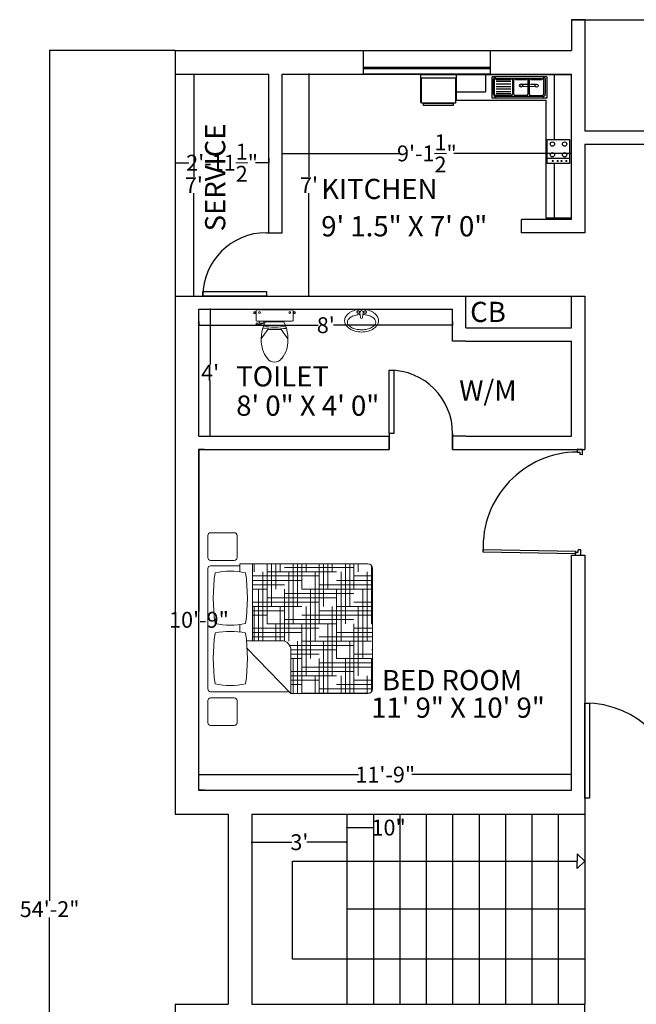
# Model space of a CAD drawing. Units: inches. Extents: x -113 to 5399, y -1393 to 3302.
# Tile 15 of 40: x 1545 to 1779, y 426 to 798. Entities that reach past the tile are written whole.
import ezdxf

# ---------------------------------------------------------------- set-up
doc = ezdxf.new("R2010")
doc.units = ezdxf.units.IN
doc.header["$MEASUREMENT"] = 0
for name, color, linetype, lineweight in [('A-ANNO-DIMS', 254, 'Continuous', 18), ('A-AREA-IDEN', 4, 'Continuous', 18), ('A-FLOR-CASE', 8, 'Continuous', 18), ('A-FLOR-FIXT', 8, 'Continuous', 18), ('doors', 2, 'Continuous', 25), ('DT TEXT', 4, 'Continuous', 18), ('furniture', 131, 'Continuous', 18), ('stairs', 210, 'Continuous', 25), ('walls', 1, 'Continuous', 25), ('windows', 3, 'Continuous', 25)]:
    doc.layers.add(name, color=color, linetype=linetype, lineweight=lineweight)
doc.layers.add('TEFRIŞ', color=11, linetype='Continuous')
doc.styles.get("Standard").update_dxf_attribs({"font": 'arial.ttf'})
doc.dimstyles.get("Standard").update_dxf_attribs({"dimtxt": 6, "dimasz": 0.18, "dimexe": 0.18, "dimexo": 0.0625, "dimgap": 0.09, "dimtad": 0, "dimtih": 1, "dimtoh": 1, "dimdec": 1, "dimzin": 0, "dimdsep": 46, "dimlunit": 4, "dimtxsty": 'Standard', "dimblk": 'ARCHTICK', "dimcen": 0.09, "dimadec": 0, "dimazin": 0, "dimtfac": 1, "dimtdec": 1, "dimtofl": 0, "dimtmove": 0, "dimatfit": 3, "dimfxl": 1, "dimtolj": 1, "dimtzin": 0, "dimarcsym": 0})

# ---------------------------------------------------------------- blocks, each defined once
blk = doc.blocks.new('*U2')
for p, q in [((0, 0), (0, -6)), ((24, 0), (24, -6))]:
    blk.add_line(p, q)
blk.add_lwpolyline([(0, 0), (0, 24), (1.75, 24), (1.75, 0)], close=True)
blk.add_arc((0, 0), 24, 0, 90)
blk = doc.blocks.new('*U3')
for p, q in [((0, 0), (0, -6)), ((36, 0), (36, -6))]:
    blk.add_line(p, q)
blk.add_lwpolyline([(0, 0), (0, 36), (1.75, 36), (1.75, 0)], close=True)
blk.add_arc((0, 0), 36, 0, 90)
blk = doc.blocks.new('*X4')
at = {"color": 0}
for p, q in [((4.359, 18.562), (4.359, 18.646)), ((4.5, 18), (4.5, 18.646)), ((4.547, 18.188), (4.547, 18.646)), ((4.594, 18.375), (4.594, 18.646)), ((4.641, 18.562), (4.641, 18.646)), ((4.781, 18), (4.781, 18.646)), ((4.828, 18.188), (4.828, 18.646)), ((4.875, 18.375), (4.875, 18.646)), ((4.922, 18.562), (4.922, 18.646)), ((5.062, 18), (5.062, 18.646)), ((5.109, 18.188), (5.109, 18.646)), ((5.156, 18.375), (5.156, 18.646)), ((5.203, 18.562), (5.203, 18.646)), ((5.344, 18), (5.344, 18.646)), ((5.391, 18.188), (5.391, 18.646)), ((5.437, 18.375), (5.437, 18.646)), ((5.484, 18.562), (5.484, 18.646)), ((5.625, 18), (5.625, 18.629)), ((4.34, 18.516), (5.062, 18.516)), ((4.453, 17.817), (4.453, 18.562)), ((4.5, 18.562), (5.25, 18.562)), ((4.687, 18.609), (5.437, 18.609)), ((4.734, 17.812), (4.734, 18.562)), ((5.016, 17.812), (5.016, 18.562)), ((5.297, 17.812), (5.297, 18.562)), ((5.437, 18.516), (5.637, 18.516)), ((5.578, 17.812), (5.578, 18.562)), ((5.625, 18.562), (5.637, 18.562)), ((4.34, 18.469), (4.875, 18.469)), ((4.34, 18.422), (4.687, 18.422)), ((5.062, 18.422), (5.637, 18.422)), ((5.25, 18.469), (5.637, 18.469)), ((4.34, 18.375), (4.5, 18.375)), ((4.406, 17.817), (4.406, 18.375)), ((4.687, 18.328), (5.437, 18.328)), ((4.687, 17.811), (4.687, 18.375)), ((4.875, 18.375), (5.625, 18.375)), ((4.969, 17.625), (4.969, 18.375)), ((5.25, 17.625), (5.25, 18.375)), ((5.531, 17.625), (5.531, 18.375)), ((4.34, 18.234), (5.062, 18.234)), ((4.5, 18.281), (5.25, 18.281)), ((5.437, 18.234), (5.637, 18.234)), ((5.625, 18.281), (5.637, 18.281)), ((4.34, 18.188), (4.875, 18.188)), ((4.34, 18.141), (4.687, 18.141)), ((4.34, 18.094), (4.5, 18.094)), ((4.359, 17.817), (4.359, 18.188)), ((4.641, 17.817), (4.641, 18.188)), ((4.875, 18.094), (5.625, 18.094)), ((4.922, 17.438), (4.922, 18.188)), ((5.062, 18.141), (5.637, 18.141)), ((5.203, 17.438), (5.203, 18.188)), ((5.25, 18.188), (5.637, 18.188)), ((5.484, 17.438), (5.484, 18.188)), ((4.5, 18), (5.25, 18)), ((4.594, 17.817), (4.594, 18)), ((4.687, 18.047), (5.437, 18.047)), ((4.875, 17.25), (4.875, 18)), ((5.156, 17.25), (5.156, 18)), ((5.437, 17.25), (5.437, 18)), ((5.625, 18), (5.637, 18)), ((4.34, 17.953), (5.062, 17.953)), ((4.34, 17.906), (4.875, 17.906)), ((5.25, 17.906), (5.637, 17.906)), ((5.437, 17.953), (5.637, 17.953)), ((4.34, 17.859), (4.687, 17.859)), ((4.828, 17.246), (4.828, 17.812)), ((4.875, 17.812), (5.625, 17.812)), ((5.062, 17.859), (5.637, 17.859)), ((5.109, 17.246), (5.109, 17.812)), ((5.391, 17.246), (5.391, 17.812)), ((4.742, 17.766), (5.437, 17.766)), ((4.755, 17.719), (5.25, 17.719)), ((4.755, 17.672), (5.062, 17.672)), ((5.437, 17.672), (5.637, 17.672)), ((5.625, 17.719), (5.637, 17.719)), ((4.755, 17.625), (4.875, 17.625)), ((4.781, 17.246), (4.781, 17.625)), ((5.062, 17.246), (5.062, 17.625)), ((5.062, 17.578), (5.637, 17.578)), ((5.25, 17.625), (5.637, 17.625)), ((5.344, 17.246), (5.344, 17.625)), ((5.625, 17.263), (5.625, 17.625)), ((4.755, 17.484), (5.437, 17.484)), ((4.875, 17.531), (5.625, 17.531)), ((4.755, 17.438), (5.25, 17.438)), ((4.755, 17.391), (5.062, 17.391)), ((4.755, 17.344), (4.875, 17.344)), ((5.016, 17.246), (5.016, 17.438)), ((5.25, 17.344), (5.637, 17.344)), ((5.297, 17.246), (5.297, 17.438)), ((5.437, 17.391), (5.637, 17.391)), ((5.578, 17.246), (5.578, 17.438)), ((5.625, 17.438), (5.637, 17.438)), ((4.875, 17.25), (5.608, 17.25)), ((4.969, 17.246), (4.969, 17.25)), ((5.062, 17.297), (5.637, 17.297)), ((5.25, 17.246), (5.25, 17.25)), ((5.531, 17.246), (5.531, 17.25))]:
    blk.add_line(p, q, dxfattribs=at)
blk = doc.blocks.new('MAT-P01')
for p, q in [((-0.021, 0.816), (-0.021, 0.56)), ((0.009, 0.846), (0.247, 0.846)), ((0.277, 0.816), (0.277, 0.56)), ((0.344, 0.816), (0.344, -0.032)), ((0.374, 0.846), (1.674, 0.846)), ((1.704, 0.816), (1.704, 0.5)), ((1.762, 0.816), (1.762, 0.56)), ((1.792, 0.846), (2.031, 0.846)), ((2.061, 0.816), (2.061, 0.56)), ((0.009, 0.53), (0.247, 0.53)), ((0.895, 0.429), (0.895, 0.049)), ((0.988, 0.5), (1.069, 0.5)), ((1.639, 0.5), (1.724, 0.5)), ((1.724, 0.5), (1.724, -0.884)), ((1.792, 0.53), (2.031, 0.53)), ((0.815, 0.423), (0.324, -0.051)), ((0.895, 0.364), (1.724, 0.364)), ((0.895, 0.364), (0.895, 0.049)), ((0.895, 0.364), (1.724, 0.364)), ((1.724, 0.364), (1.724, -0.884)), ((0.324, -0.051), (0.795, -0.051)), ((0.324, -0.051), (0.324, -0.884)), ((0.374, -0.934), (1.674, -0.934))]:
    blk.add_line(p, q)
for centre, radius, start, end in [((0.009, 0.816), 0.03, 90, 180), ((0.247, 0.816), 0.03, 0, 90), ((0.374, 0.816), 0.03, 90, 180), ((1.225, 0.603), 0.814, 168.373, 191.627), ((0.703, -1.144), 1.931, 81.8162, 98.1838), ((0.181, 0.603), 0.814, 348.373, 11.627), ((1.877, 0.603), 0.814, 168.373, 191.627), ((1.354, -1.144), 1.931, 81.8162, 98.1838), ((0.832, 0.603), 0.814, 348.373, 11.627), ((1.674, 0.816), 0.03, 0, 90), ((1.792, 0.816), 0.03, 90, 180), ((2.031, 0.816), 0.03, 0, 90), ((0.009, 0.56), 0.03, 180, 270), ((0.247, 0.56), 0.03, 270, 0), ((1.792, 0.56), 0.03, 180, 270), ((2.031, 0.56), 0.03, 270, 0), ((0.703, 2.35), 1.931, 261.8162, 278.1838), ((1.354, 2.35), 1.931, 261.8162, 278.1838), ((0.795, 0.049), 0.1, 270, 0), ((0.374, -0.884), 0.05, 180, 270), ((1.674, -0.884), 0.05, 270, 0)]:
    blk.add_arc(centre, radius, start, end)
at = {"rotation": 270}
blk.add_blockref('*X4', (-16.922, 4.704), dxfattribs=at)
blk = doc.blocks.new('A$C008029BD')
at = {"layer": 'TEFRIŞ', "ltscale": 0.05}
for p, q in [((0, 0), (0, -3.55)), ((3.37, 0), (0, 0)), ((3.37, 0), (3.37, -0.6)), ((1.522, -0.4), (0, -0.4)), ((3.37, -0.4), (2.083, -0.4)), ((0.05, -0.581), (0.05, -1.869)), ((0.05, -0.581), (0.55, -0.581)), ((0.086, -1.773), (0.086, -0.677)), ((0.096, -0.617), (0.454, -0.617)), ((0.099, -0.659), (0.457, -0.659)), ((0.514, -0.677), (0.514, -1.773)), ((0.55, -0.581), (0.55, -1.869)), ((0.6, -2.71), (0.6, -0.6)), ((3.37, -0.6), (0.6, -0.6)), ((0.113, -0.954), (0.113, -0.695)), ((0.23, -0.846), (0.229, -0.967)), ((0.28, -0.846), (0.277, -1.158)), ((0.493, -0.695), (0.493, -0.954)), ((0.096, -1.024), (0.454, -1.024)), ((0.457, -0.99), (0.099, -0.99)), ((0.11, -1.319), (0.11, -1.06)), ((0.228, -1.02), (0.227, -1.159)), ((0.49, -1.06), (0.49, -1.319)), ((0.454, -1.355), (0.096, -1.355)), ((0.096, -1.391), (0.454, -1.391)), ((0.11, -1.773), (0.11, -1.427)), ((0.154, -1.773), (0.154, -1.427)), ((0.214, -1.773), (0.214, -1.427)), ((0.274, -1.773), (0.274, -1.427)), ((0.334, -1.773), (0.334, -1.427)), ((0.39, -1.773), (0.39, -1.427)), ((0.444, -1.773), (0.444, -1.427)), ((0.49, -1.427), (0.49, -1.773)), ((0.454, -1.809), (0.096, -1.809)), ((0.454, -1.833), (0.096, -1.833)), ((0, -2.025), (0.4, -2.025)), ((0.55, -1.869), (0.05, -1.869)), ((0.4, -2.71), (0.4, -2.025)), ((0, -2.71), (0.6, -2.71)), ((0, -3.55), (0.65, -3.55))]:
    blk.add_line(p, q, dxfattribs=at)
at = {"layer": 'TEFRIŞ'}
blk.add_line((1.969, -0.05), (1.969, -0.572), dxfattribs=at)
at = {"layer": 'TEFRIŞ', "ltscale": 0.05}
for points in [[(1.522, -0.05), (2.083, -0.05), (2.083, -0.572), (1.522, -0.572)], [(0.67, -2.73), (0.67, -3.53), (0.07, -3.53), (0.07, -2.73)], [(0.72, -2.78), (0.72, -3.48), (0.67, -3.48), (0.67, -2.78)]]:
    blk.add_lwpolyline(points, close=True, dxfattribs=at)
at = {"layer": 'TEFRIŞ', "const_width": 0.025}
for points in [[(2.014, -0.123, 1), (2.039, -0.123, 1)], [(2.014, -0.236, 1), (2.039, -0.236, 1)], [(2.014, -0.327, 1), (2.039, -0.327, 1)], [(2.014, -0.44, 1), (2.039, -0.44, 1)]]:
    blk.add_lwpolyline(points, format="xyb", close=True, dxfattribs=at)
at = {"layer": 'TEFRIŞ', "ltscale": 0.05}
for centre, radius in [((1.628, -0.164), 0.0505), ((1.628, -0.45), 0.0505), ((0.255, -0.82), 0.036), ((0.252, -1.184), 0.036)]:
    blk.add_circle(centre, radius, dxfattribs=at)
at = {"layer": 'TEFRIŞ'}
for centre in [(1.88, -0.164), (1.88, -0.45)]:
    blk.add_circle(centre, 0.0505, dxfattribs=at)
at = {"layer": 'TEFRIŞ', "ltscale": 0.05}
for centre, radius, start, end in [((0.108, -0.649), 0.0351, 110.4976, 230.5777), ((0.118, -0.673), 0.023, 143.9853, 258.5157), ((0.454, -0.677), 0.06, 0, 90), ((0.457, -0.695), 0.036, 0, 90), ((0.115, -1.038), 0.023, 143.9853, 258.5157), ((0.118, -0.976), 0.023, 101.4843, 216.0147), ((0.454, -1.06), 0.036, 0, 90), ((0.457, -0.954), 0.036, 270, 0), ((0.115, -1.341), 0.023, 101.4843, 216.0147), ((0.454, -1.319), 0.036, 270, 0), ((0.115, -1.405), 0.023, 143.9853, 258.5157), ((0.454, -1.427), 0.036, 0, 90), ((0.108, -1.801), 0.0351, 129.4223, 249.5024), ((0.115, -1.796), 0.023, 101.4843, 216.0147), ((0.454, -1.773), 0.06, 270, 0), ((0.454, -1.773), 0.036, 270, 0)]:
    blk.add_arc(centre, radius, start, end, dxfattribs=at)
blk = doc.blocks.new('toilet-3')
at = {"color": 0, "linetype": 'ByBlock'}
for p, q in [((-0.281, -0.05), (-0.281, -0.069)), ((-0.281, -0.05), (-0.261, -0.05)), ((-0.281, -0.069), (-0.261, -0.069)), ((-0.261, -0.047), (-0.261, -0.072)), ((-0.261, -0.047), (-0.251, -0.047)), ((-0.261, -0.072), (-0.251, -0.072)), ((-0.251, -0.047), (-0.251, -0.072)), ((-0.25, -0.03), (-0.25, -0.165)), ((0.24, -0.02), (-0.24, -0.02)), ((0.25, -0.03), (0.25, -0.165)), ((0.261, -0.047), (0.251, -0.047)), ((0.251, -0.047), (0.251, -0.072)), ((0.261, -0.072), (0.251, -0.072)), ((0.261, -0.047), (0.261, -0.072)), ((0.281, -0.05), (0.261, -0.05)), ((0.281, -0.069), (0.261, -0.069)), ((0.281, -0.05), (0.281, -0.069)), ((-0.144, -0.2), (-0.25, -0.2)), ((-0.25, -0.2), (-0.25, -0.222)), ((-0.198, -0.222), (-0.25, -0.222)), ((0.24, -0.175), (-0.24, -0.175)), ((-0.202, -0.2), (-0.202, -0.175)), ((-0.198, -0.222), (-0.16, -0.207)), ((-0.16, -0.207), (-0.16, -0.2)), ((-0.144, -0.2), (-0.144, -0.175)), ((0.125, -0.182), (-0.125, -0.182)), ((-0.089, -0.287), (-0.18, -0.415)), ((0.089, -0.287), (-0.089, -0.287)), ((0.089, -0.287), (0.18, -0.415))]:
    blk.add_line(p, q, dxfattribs=at)
for centre in [(-0.205, -0.059), (0.205, -0.059)]:
    blk.add_circle(centre, 0.0125, dxfattribs=at)
for centre, radius, start, end in [((-0.24, -0.03), 0.01, 90, 180), ((0.24, -0.03), 0.01, 0, 90), ((-0.24, -0.165), 0.01, 180, 270), ((0.376, -0.424), 0.557, 154.2321, 193.6755), ((-0.013, -1.787), 1.521, 83.4552, 95.5271), ((-0.005, -0.896), 0.659, 75.9276, 103.0204), ((-0.376, -0.424), 0.557, 346.3245, 25.7679), ((0.24, -0.165), 0.01, 270, 0), ((0.262, -0.406), 0.452, 199.2942, 217.2549), ((-0.265, -0.4), 0.457, 322.2382, 340.1051), ((-0.001, -0.609), 0.12, 216.3794, 323.6206)]:
    blk.add_arc(centre, radius, start, end, dxfattribs=at)
blk = doc.blocks.new('wash-6')
at = {"color": 0, "linetype": 'ByBlock'}
for p, q in [((-0.036, -0.063), (-0.021, -0.18)), ((0.036, -0.063), (0.021, -0.18))]:
    blk.add_line(p, q, dxfattribs=at)
for centre, radius in [((-0.075, -0.062), 0.0325), ((-0.075, -0.062), 0.0263), ((0.075, -0.062), 0.0325), ((0.075, -0.062), 0.0263)]:
    blk.add_circle(centre, radius, dxfattribs=at)
for centre, radius, start, end in [((0, -0.56), 0.56, 90, 105.4371), ((-0.204, -0.25), 0.17, 148.1465, 180), ((-0.107, -0.311), 0.285, 123.6901, 148.1465), ((-0.114, -0.361), 0.225, 118.369, 142.5096), ((-0.042, -0.407), 0.401, 105.4371, 123.6901), ((-0.045, -0.488), 0.37, 102.6081, 118.369), ((0, -0.69), 0.576, 92.9466, 102.6081), ((0, -0.063), 0.0361, 0, 180), ((0, -0.18), 0.0215, 180, 0), ((0, -0.56), 0.56, 74.5629, 90), ((0, -0.69), 0.576, 77.3919, 87.0534), ((0.045, -0.488), 0.37, 61.631, 77.3919), ((0.042, -0.407), 0.401, 56.3099, 74.5629), ((0.114, -0.361), 0.225, 37.4904, 61.631), ((0.107, -0.311), 0.285, 31.8535, 56.3099), ((0.204, -0.25), 0.17, 0, 31.8535), ((-0.204, -0.25), 0.17, 180, 211.8535), ((-0.107, -0.189), 0.285, 211.8535, 236.3099), ((-0.217, -0.282), 0.0954, 142.5096, 180), ((-0.217, -0.282), 0.0954, 180, 217.4904), ((-0.114, -0.203), 0.225, 217.4904, 241.631), ((-0.042, -0.092), 0.401, 236.3099, 254.5629), ((-0.045, -0.076), 0.37, 241.631, 257.3919), ((0.045, -0.076), 0.37, 282.6081, 298.369), ((0.042, -0.092), 0.401, 285.4371, 303.6901), ((0.114, -0.203), 0.225, 298.369, 322.5096), ((0.107, -0.189), 0.285, 303.6901, 328.1465), ((0.217, -0.282), 0.0954, 0, 37.4904), ((0.217, -0.282), 0.0954, 322.5096, 0), ((0.204, -0.25), 0.17, 328.1465, 0), ((0, 0.06), 0.56, 254.5629, 270), ((0, 0.125), 0.576, 257.3919, 270), ((0, 0.125), 0.576, 270, 282.6081), ((0, 0.06), 0.56, 270, 285.4371)]:
    blk.add_arc(centre, radius, start, end, dxfattribs=at)
blk = doc.blocks.new('_ArchTick')
at = {"color": 0, "linetype": 'ByBlock', "const_width": 0.15}
blk.add_lwpolyline([(-0.5, -0.5), (0.5, 0.5)], dxfattribs=at)
blk = doc.blocks.new('*D52')
at = {"layer": 'A-ANNO-DIMS', "color": 0, "lineweight": -2, "transparency": 16777216}
for p, q in [((1655.07, 777.53), (1654.71, 777.53)), ((1654.89, 777.53), (1654.89, 738.62)), ((1654.89, 693.53), (1654.89, 732.44)), ((1655.07, 693.53), (1654.71, 693.53))]:
    blk.add_line(p, q, dxfattribs=at)
at = {"layer": 'Defpoints', "color": 0, "transparency": 16777216}
for p in [(1655.13, 777.53), (1654.89, 693.53), (1655.13, 693.53)]:
    blk.add_point(p, dxfattribs=at)
at = {"layer": 'A-ANNO-DIMS', "color": 0, "lineweight": -2, "transparency": 16777216, "xscale": 0.18, "yscale": 0.18, "zscale": 0.18}
for p, rotation in [((1654.89, 777.53), 90), ((1654.89, 693.53), 270)]:
    blk.add_blockref('_ArchTick', p, dxfattribs=dict(at, rotation=rotation))
at = {"layer": 'A-ANNO-DIMS', "color": 0, "transparency": 16777216, "insert": (1654.89, 735.53), "char_height": 6, "attachment_point": 5}
blk.add_mtext("\\A1;7'", dxfattribs=at)
blk = doc.blocks.new('*D53')
at = {"layer": 'A-ANNO-DIMS', "color": 0, "lineweight": -2, "transparency": 16777216}
for p, q in [((1644.76, 747.53), (1689.26, 747.53)), ((1644.76, 747.47), (1644.76, 747.35)), ((1754.26, 747.53), (1709.76, 747.53)), ((1754.26, 747.59), (1754.26, 747.71))]:
    blk.add_line(p, q, dxfattribs=at)
at = {"layer": 'Defpoints', "color": 0, "transparency": 16777216}
for p in [(1644.76, 747.53), (1754.26, 747.53), (1754.26, 747.53)]:
    blk.add_point(p, dxfattribs=at)
at = {"layer": 'A-ANNO-DIMS', "color": 0, "lineweight": -2, "transparency": 16777216, "xscale": 0.18, "yscale": 0.18, "zscale": 0.18, "rotation": 180}
blk.add_blockref('_ArchTick', (1644.76, 747.53), dxfattribs=at)
at = {"layer": 'A-ANNO-DIMS', "color": 0, "lineweight": -2, "transparency": 16777216, "xscale": 0.18, "yscale": 0.18, "zscale": 0.18}
blk.add_blockref('_ArchTick', (1754.26, 747.53), dxfattribs=at)
at = {"layer": 'A-ANNO-DIMS', "color": 0, "transparency": 16777216, "insert": (1699.51, 747.53), "char_height": 6, "attachment_point": 5}
blk.add_mtext('\\A1;9\'-1{\\H1x;\\S1/2;}"', dxfattribs=at)
blk = doc.blocks.new('*D60')
at = {"layer": 'A-ANNO-DIMS', "color": 0, "lineweight": -2, "transparency": 16777216}
for p, q in [((1604.2, 786.53), (1556.55, 786.53)), ((1556.73, 786.53), (1556.73, 464.69)), ((1556.73, 136.53), (1556.73, 458.38)), ((1604.2, 136.53), (1556.55, 136.53))]:
    blk.add_line(p, q, dxfattribs=at)
at = {"layer": 'Defpoints', "color": 0, "transparency": 16777216}
for p in [(1604.26, 786.53), (1556.73, 136.53), (1604.26, 136.53)]:
    blk.add_point(p, dxfattribs=at)
at = {"layer": 'A-ANNO-DIMS', "color": 0, "lineweight": -2, "transparency": 16777216, "xscale": 0.18, "yscale": 0.18, "zscale": 0.18}
for p, rotation in [((1556.73, 786.53), 90), ((1556.73, 136.53), 270)]:
    blk.add_blockref('_ArchTick', p, dxfattribs=dict(at, rotation=rotation))
at = {"layer": 'A-ANNO-DIMS', "color": 0, "transparency": 16777216, "insert": (1556.73, 461.53), "char_height": 6, "attachment_point": 5}
blk.add_mtext('\\A1;54\'-2"', dxfattribs=at)
blk = doc.blocks.new('*D69')
at = {"layer": 'A-ANNO-DIMS', "color": 0, "lineweight": -2, "transparency": 16777216}
for p, q in [((1633.26, 486.55), (1633.26, 487.06)), ((1633.26, 486.88), (1648.41, 486.88)), ((1669.26, 486.88), (1654.11, 486.88)), ((1669.26, 486.55), (1669.26, 487.06))]:
    blk.add_line(p, q, dxfattribs=at)
at = {"layer": 'Defpoints', "color": 0, "transparency": 16777216}
for p in [(1633.26, 486.49), (1669.26, 486.88), (1669.26, 486.49)]:
    blk.add_point(p, dxfattribs=at)
at = {"layer": 'A-ANNO-DIMS', "color": 0, "lineweight": -2, "transparency": 16777216, "xscale": 0.18, "yscale": 0.18, "zscale": 0.18, "rotation": 180}
blk.add_blockref('_ArchTick', (1633.26, 486.88), dxfattribs=at)
at = {"layer": 'A-ANNO-DIMS', "color": 0, "lineweight": -2, "transparency": 16777216, "xscale": 0.18, "yscale": 0.18, "zscale": 0.18}
blk.add_blockref('_ArchTick', (1669.26, 486.88), dxfattribs=at)
at = {"layer": 'A-ANNO-DIMS', "color": 0, "transparency": 16777216, "insert": (1651.26, 486.88), "char_height": 6, "attachment_point": 5}
blk.add_mtext("\\A1;3'", dxfattribs=at)
blk = doc.blocks.new('*D70')
at = {"layer": 'A-ANNO-DIMS', "color": 0, "lineweight": -2, "transparency": 16777216}
for p, q in [((1669.26, 492.47), (1669.26, 492.59)), ((1669.26, 492.41), (1679.26, 492.41)), ((1679.26, 492.47), (1679.26, 492.59)), ((1679.26, 492.41), (1679.44, 492.41))]:
    blk.add_line(p, q, dxfattribs=at)
at = {"layer": 'Defpoints', "color": 0, "transparency": 16777216}
for p in [(1669.26, 492.41), (1679.26, 492.41), (1679.26, 492.41)]:
    blk.add_point(p, dxfattribs=at)
at = {"layer": 'A-ANNO-DIMS', "color": 0, "lineweight": -2, "transparency": 16777216, "xscale": 0.18, "yscale": 0.18, "zscale": 0.18, "rotation": 180}
blk.add_blockref('_ArchTick', (1669.26, 492.41), dxfattribs=at)
at = {"layer": 'A-ANNO-DIMS', "color": 0, "lineweight": -2, "transparency": 16777216, "xscale": 0.18, "yscale": 0.18, "zscale": 0.18}
blk.add_blockref('_ArchTick', (1679.26, 492.41), dxfattribs=at)
at = {"layer": 'A-ANNO-DIMS', "color": 0, "transparency": 16777216, "insert": (1685.03, 492.41), "char_height": 6, "attachment_point": 5}
blk.add_mtext('\\A1;10"', dxfattribs=at)
blk = doc.blocks.new('*D71')
at = {"layer": 'A-ANNO-DIMS', "color": 0, "lineweight": -2, "transparency": 16777216}
for p, q in [((1615.35, 635.53), (1613.08, 635.53)), ((1613.26, 635.53), (1613.26, 574.19)), ((1613.26, 506.53), (1613.26, 567.88)), ((1615.35, 506.53), (1613.08, 506.53))]:
    blk.add_line(p, q, dxfattribs=at)
at = {"layer": 'Defpoints', "color": 0, "transparency": 16777216}
for p in [(1615.42, 635.53), (1613.26, 506.53), (1615.42, 506.53)]:
    blk.add_point(p, dxfattribs=at)
at = {"layer": 'A-ANNO-DIMS', "color": 0, "lineweight": -2, "transparency": 16777216, "xscale": 0.18, "yscale": 0.18, "zscale": 0.18}
for p, rotation in [((1613.26, 635.53), 90), ((1613.26, 506.53), 270)]:
    blk.add_blockref('_ArchTick', p, dxfattribs=dict(at, rotation=rotation))
at = {"layer": 'A-ANNO-DIMS', "color": 0, "transparency": 16777216, "insert": (1613.26, 571.03), "char_height": 6, "attachment_point": 5}
blk.add_mtext('\\A1;10\'-9"', dxfattribs=at)
blk = doc.blocks.new('*D72')
at = {"layer": 'A-ANNO-DIMS', "color": 0, "lineweight": -2, "transparency": 16777216}
for p, q in [((1613.26, 512.2), (1613.26, 512.64)), ((1613.26, 512.46), (1673.65, 512.46)), ((1754.26, 512.46), (1693.88, 512.46)), ((1754.26, 512.2), (1754.26, 512.64))]:
    blk.add_line(p, q, dxfattribs=at)
at = {"layer": 'Defpoints', "color": 0, "transparency": 16777216}
for p in [(1613.26, 512.46), (1613.26, 512.13), (1754.26, 512.13)]:
    blk.add_point(p, dxfattribs=at)
at = {"layer": 'A-ANNO-DIMS', "color": 0, "lineweight": -2, "transparency": 16777216, "xscale": 0.18, "yscale": 0.18, "zscale": 0.18, "rotation": 180}
blk.add_blockref('_ArchTick', (1613.26, 512.46), dxfattribs=at)
at = {"layer": 'A-ANNO-DIMS', "color": 0, "lineweight": -2, "transparency": 16777216, "xscale": 0.18, "yscale": 0.18, "zscale": 0.18}
blk.add_blockref('_ArchTick', (1754.26, 512.46), dxfattribs=at)
at = {"layer": 'A-ANNO-DIMS', "color": 0, "transparency": 16777216, "insert": (1683.76, 512.46), "char_height": 6, "attachment_point": 5}
blk.add_mtext('\\A1;11\'-9"', dxfattribs=at)
blk = doc.blocks.new('*D73')
at = {"layer": 'A-ANNO-DIMS', "color": 0, "lineweight": -2, "transparency": 16777216}
for p, q in [((1617.61, 688.53), (1617.32, 688.53)), ((1617.5, 688.53), (1617.5, 667.62)), ((1617.5, 640.53), (1617.5, 661.44)), ((1617.61, 640.53), (1617.32, 640.53))]:
    blk.add_line(p, q, dxfattribs=at)
at = {"layer": 'Defpoints', "color": 0, "transparency": 16777216}
for p in [(1617.68, 688.53), (1617.5, 640.53), (1617.68, 640.53)]:
    blk.add_point(p, dxfattribs=at)
at = {"layer": 'A-ANNO-DIMS', "color": 0, "lineweight": -2, "transparency": 16777216, "xscale": 0.18, "yscale": 0.18, "zscale": 0.18}
for p, rotation in [((1617.5, 688.53), 90), ((1617.5, 640.53), 270)]:
    blk.add_blockref('_ArchTick', p, dxfattribs=dict(at, rotation=rotation))
at = {"layer": 'A-ANNO-DIMS', "color": 0, "transparency": 16777216, "insert": (1617.5, 664.53), "char_height": 6, "attachment_point": 5}
blk.add_mtext("\\A1;4'", dxfattribs=at)
blk = doc.blocks.new('*D74')
at = {"layer": 'A-ANNO-DIMS', "color": 0, "lineweight": -2, "transparency": 16777216}
for p, q in [((1613.26, 683.87), (1613.26, 682.35)), ((1613.26, 682.53), (1658.41, 682.53)), ((1709.26, 682.53), (1664.12, 682.53)), ((1709.26, 683.87), (1709.26, 682.35))]:
    blk.add_line(p, q, dxfattribs=at)
at = {"layer": 'Defpoints', "color": 0, "transparency": 16777216}
for p in [(1613.26, 683.93), (1709.26, 683.93), (1709.26, 682.53)]:
    blk.add_point(p, dxfattribs=at)
at = {"layer": 'A-ANNO-DIMS', "color": 0, "lineweight": -2, "transparency": 16777216, "xscale": 0.18, "yscale": 0.18, "zscale": 0.18, "rotation": 180}
blk.add_blockref('_ArchTick', (1613.26, 682.53), dxfattribs=at)
at = {"layer": 'A-ANNO-DIMS', "color": 0, "lineweight": -2, "transparency": 16777216, "xscale": 0.18, "yscale": 0.18, "zscale": 0.18}
blk.add_blockref('_ArchTick', (1709.26, 682.53), dxfattribs=at)
at = {"layer": 'A-ANNO-DIMS', "color": 0, "transparency": 16777216, "insert": (1661.26, 682.53), "char_height": 6, "attachment_point": 5}
blk.add_mtext("\\A1;8'", dxfattribs=at)
blk = doc.blocks.new('*D75')
at = {"layer": 'A-ANNO-DIMS', "color": 0, "lineweight": -2, "transparency": 16777216}
for p, q in [((1604.26, 745.69), (1604.26, 743.83)), ((1639.76, 745.69), (1639.76, 743.83)), ((1604.26, 744.01), (1609.38, 744.01)), ((1639.76, 744.01), (1634.65, 744.01))]:
    blk.add_line(p, q, dxfattribs=at)
at = {"layer": 'Defpoints', "color": 0, "transparency": 16777216}
for p in [(1604.26, 745.76), (1639.76, 745.76), (1639.76, 744.01)]:
    blk.add_point(p, dxfattribs=at)
at = {"layer": 'A-ANNO-DIMS', "color": 0, "lineweight": -2, "transparency": 16777216, "xscale": 0.18, "yscale": 0.18, "zscale": 0.18, "rotation": 180}
blk.add_blockref('_ArchTick', (1604.26, 744.01), dxfattribs=at)
at = {"layer": 'A-ANNO-DIMS', "color": 0, "lineweight": -2, "transparency": 16777216, "xscale": 0.18, "yscale": 0.18, "zscale": 0.18}
blk.add_blockref('_ArchTick', (1639.76, 744.01), dxfattribs=at)
at = {"layer": 'A-ANNO-DIMS', "color": 0, "transparency": 16777216, "insert": (1622.01, 744.01), "char_height": 6, "attachment_point": 5}
blk.add_mtext('\\A1;2\'-11{\\H1x;\\S1/2;}"', dxfattribs=at)
blk = doc.blocks.new('*D76')
at = {"layer": 'A-ANNO-DIMS', "color": 0, "lineweight": -2, "transparency": 16777216}
for p, q in [((1609.38, 777.53), (1611.51, 777.53)), ((1611.33, 777.53), (1611.33, 738.62)), ((1611.33, 693.53), (1611.33, 732.44)), ((1609.38, 693.53), (1611.51, 693.53))]:
    blk.add_line(p, q, dxfattribs=at)
at = {"layer": 'Defpoints', "color": 0, "transparency": 16777216}
for p in [(1609.31, 777.53), (1609.31, 693.53), (1611.33, 693.53)]:
    blk.add_point(p, dxfattribs=at)
at = {"layer": 'A-ANNO-DIMS', "color": 0, "lineweight": -2, "transparency": 16777216, "xscale": 0.18, "yscale": 0.18, "zscale": 0.18}
for p, rotation in [((1611.33, 777.53), 90), ((1611.33, 693.53), 270)]:
    blk.add_blockref('_ArchTick', p, dxfattribs=dict(at, rotation=rotation))
at = {"layer": 'A-ANNO-DIMS', "color": 0, "transparency": 16777216, "insert": (1611.33, 735.53), "char_height": 6, "attachment_point": 5}
blk.add_mtext("\\A1;7'", dxfattribs=at)
blk = doc.blocks.new('WIN-PLAN-48IN')
h = blk.add_hatch(color=256)
h.dxf.hatch_style = 1
h.paths.add_polyline_path([(48, 2.5), (0, 2.5), (0, 2), (48, 2)])
for p, q in [((0, 9), (48, 9)), ((0, 0), (0, 9)), ((48, 9), (48, 0)), ((48, 2.5), (0, 2.5)), ((48, 2), (0, 2)), ((48, 0), (0, 0))]:
    blk.add_line(p, q)
blk = doc.blocks.new('DOOR-SINGLE-36IN-PLAN')
for p, q in [((0.5, 2), (0.5, 36.98)), ((0.5, 36.98), (1.5, 36.98)), ((1.5, 36.98), (1.5, 2)), ((0, 2), (0, 0)), ((0, 2), (1.04, 2)), ((1.5, 2), (0.5, 2)), ((1.04, 2), (1.04, 0.98)), ((1.04, 0.98), (2, 0.98)), ((2, 0), (2, 0.98)), ((38.96, 0.98), (38, 0.98)), ((38, 0), (38, 0.98)), ((40, 2), (38.96, 2)), ((38.96, 2), (38.96, 0.98)), ((40, 0), (40, 2)), ((0, 0), (2, 0)), ((0, 0), (2, 0)), ((38, 0), (40, 0))]:
    blk.add_line(p, q)
blk.add_arc((2.94, 0.99), 36.04, 1.6003, 93.0893)
blk = doc.blocks.new('*D209')
at = {"layer": 'A-ANNO-DIMS', "color": 0, "lineweight": -2, "transparency": 16777216}
for p, q in [((1754.32, 798.03), (2074.39, 798.03)), ((2074.21, 798.03), (2074.21, 467.19)), ((2074.21, 130.03), (2074.21, 460.88)), ((1754.32, 130.03), (2074.39, 130.03))]:
    blk.add_line(p, q, dxfattribs=at)
at = {"layer": 'Defpoints', "color": 0, "transparency": 16777216}
for p in [(1754.26, 798.03), (2074.21, 798.03), (1754.26, 130.03)]:
    blk.add_point(p, dxfattribs=at)
at = {"layer": 'A-ANNO-DIMS', "color": 0, "lineweight": -2, "transparency": 16777216, "xscale": 0.18, "yscale": 0.18, "zscale": 0.18}
for p, rotation in [((2074.21, 798.03), 90), ((2074.21, 130.03), 270)]:
    blk.add_blockref('_ArchTick', p, dxfattribs=dict(at, rotation=rotation))
at = {"layer": 'A-ANNO-DIMS', "color": 0, "transparency": 16777216, "insert": (2074.21, 464.03), "char_height": 6, "attachment_point": 5}
blk.add_mtext('\\A1;55\'-8"', dxfattribs=at)

msp = doc.modelspace()

# ---------------------------------------------------------------- linework, layer by layer
at = {"layer": 'stairs'}
for p, q in [((1669.26, 497.53), (1669.26, 425.53)), ((1679.26, 497.53), (1679.26, 425.53)), ((1689.26, 497.53), (1689.26, 425.53)), ((1699.26, 497.53), (1699.26, 425.53)), ((1709.26, 497.53), (1709.26, 425.53)), ((1719.26, 497.53), (1719.26, 425.53)), ((1729.26, 497.53), (1729.26, 425.53)), ((1739.26, 497.53), (1739.26, 425.53)), ((1749.26, 497.53), (1749.26, 425.53)), ((1759.26, 497.53), (1759.26, 425.53)), ((1759.26, 479.67), (1756.34, 482.43)), ((1756.34, 482.43), (1756.34, 479.67)), ((1648.72, 442.62), (1648.72, 479.67)), ((1648.72, 479.67), (1756.34, 479.67)), ((1759.26, 479.67), (1756.34, 476.91)), ((1756.34, 476.91), (1756.34, 479.67)), ((1759.26, 461.53), (1669.26, 461.53)), ((1759.26, 442.62), (1648.72, 442.62))]:
    msp.add_line(p, q, dxfattribs=at)
at = {"layer": 'walls'}
for p, q in [((1759.26, 798.03), (1754.26, 798.03)), ((1754.26, 798.03), (1754.26, 786.53)), ((1759.26, 798.03), (1759.26, 756.03)), ((1759.26, 798.03), (1891.26, 798.03)), ((1604.26, 786.53), (1604.26, 497.53)), ((1604.26, 786.53), (1754.26, 786.53)), ((1604.26, 777.53), (1639.76, 777.53)), ((1639.76, 717.53), (1639.76, 777.53)), ((1644.76, 717.53), (1644.76, 777.53)), ((1644.76, 777.53), (1754.26, 777.53)), ((1754.26, 722.53), (1754.26, 777.53)), ((1759.26, 756.03), (1801.26, 756.03)), ((1759.26, 751.03), (1759.26, 717.53)), ((1759.26, 751.03), (1801.26, 751.03)), ((1754.26, 722.53), (1735.26, 722.53)), ((1735.26, 717.53), (1735.26, 722.53)), ((1639.76, 717.53), (1644.76, 717.53)), ((1759.26, 717.53), (1735.26, 717.53)), ((1604.26, 693.53), (1639.76, 693.53)), ((1639.76, 693.53), (1644.76, 693.53)), ((1644.76, 693.53), (1754.26, 693.53)), ((1714.26, 681.53), (1714.26, 693.53)), ((1754.26, 681.53), (1754.26, 693.53)), ((1754.26, 693.53), (1759.26, 693.53)), ((1759.26, 693.53), (1759.26, 635.53)), ((1613.26, 640.53), (1613.26, 688.53)), ((1613.26, 688.53), (1709.26, 688.53)), ((1709.26, 676.53), (1709.26, 688.53)), ((1714.26, 681.53), (1754.26, 681.53)), ((1714.26, 676.53), (1709.26, 676.53)), ((1714.26, 676.53), (1754.26, 676.53)), ((1754.26, 640.53), (1754.26, 676.53)), ((1709.26, 635.53), (1709.26, 641.53)), ((1613.26, 640.53), (1685.26, 640.53)), ((1685.26, 635.53), (1685.26, 640.53)), ((1714.26, 640.53), (1709.26, 640.53)), ((1714.26, 640.53), (1754.26, 640.53)), ((1613.26, 506.53), (1613.26, 635.53)), ((1613.26, 635.53), (1685.26, 635.53)), ((1709.26, 635.53), (1754.26, 635.53)), ((1754.26, 635.53), (1759.26, 635.53)), ((1754.26, 506.53), (1754.26, 595.53)), ((1754.26, 595.53), (1759.26, 595.53)), ((1759.26, 595.53), (1759.26, 506.53)), ((1613.26, 506.53), (1754.26, 506.53)), ((1759.26, 506.53), (1759.26, 497.53)), ((1604.26, 497.53), (1624.26, 497.53)), ((1624.26, 497.53), (1624.26, 425.53)), ((1633.26, 497.53), (1759.26, 497.53)), ((1633.26, 497.53), (1633.26, 425.53)), ((1604.26, 425.53), (1604.26, 136.53)), ((1604.26, 425.53), (1624.26, 425.53)), ((1633.26, 425.53), (1759.26, 425.53)), ((1759.26, 416.53), (1759.26, 425.53))]:
    msp.add_line(p, q, dxfattribs=at)

# ---------------------------------------------------------------- block references
at = {"layer": 'A-FLOR-CASE', "xscale": 16.09806929200166, "yscale": 16.09806929200166, "zscale": 16.09806929200166, "rotation": 270}
msp.add_blockref('A$C008029BD', (1754.26, 777.29), dxfattribs=at)
at = {"layer": 'A-FLOR-FIXT'}
for name, p, xscale, yscale, zscale in [('toilet-3', (1641.87, 688.93), 27.95492935005888, 27.95492935005888, 27.95492935005888), ('wash-6', (1674.81, 688.53), 17.16666334294967, 17.16666334294967, 17.16666334294967)]:
    msp.add_blockref(name, p, dxfattribs=dict(at, xscale=xscale, yscale=yscale, zscale=zscale))
at = {"layer": 'doors'}
for name, p, rotation in [('*U2', (1638.76, 693.53), 90.00000000000003), ('DOOR-SINGLE-36IN-PLAN', (1757.76, 595.52), 89.09244041659109)]:
    msp.add_blockref(name, p, dxfattribs=dict(at, rotation=rotation))
for name, p in [('*U2', (1685.26, 641.53)), ('*U3', (1759.26, 503.53))]:
    msp.add_blockref(name, p, dxfattribs=at)
at = {"layer": 'doors', "xscale": -1, "rotation": 180}
msp.add_blockref('*U3', (1759.26, 419.53), dxfattribs=at)
at = {"layer": 'furniture', "xscale": 35.02364872074636, "yscale": 35.02364872074636, "zscale": 35.02364872074636, "rotation": 90}
msp.add_blockref('MAT-P01', (1646.25, 531.79), dxfattribs=at)
at = {"layer": 'windows'}
msp.add_blockref('WIN-PLAN-48IN', (1675.51, 777.53), dxfattribs=at)

# ---------------------------------------------------------------- texts
at = {"layer": 'A-AREA-IDEN'}
msp.add_text('SERVICE', height=7.647, rotation=90, dxfattribs=at).set_placement((1623.22, 718.03))
for s, height, p in [('KITCHEN', 7.647, (1659.53, 730.26)), ('9\' 1.5" X 7\' 0"', 7.6473, (1659.53, 716.14)), ('TOILET', 7.647, (1627.35, 659.34)), ('8\' 0" X 4\' 0"', 7.6473, (1627.35, 648.26)), ('BED ROOM', 7.647, (1682.5, 544.39)), ('11\' 9" X 10\' 9"', 7.6473, (1678.4, 533.97))]:
    msp.add_text(s, height=height, dxfattribs=at).set_placement(p)
at = {"layer": 'DT TEXT'}
for s, p in [('CB', (1715.89, 683.72)), (' W/M', (1709.42, 653.97))]:
    msp.add_text(s, height=7.647, dxfattribs=at).set_placement(p)

# ---------------------------------------------------------------- dimensions: what is measured, and where the dimension line sits
at = {"layer": 'A-ANNO-DIMS'}
for base, p1, p2, override, picture, middle in [((2074.21, 798.03), (1754.26, 130.03), (1754.26, 798.03), {"dimdec": 1, "dimlfac": 1, "dimrnd": 0, "dimzin": 1, "dimdsep": 46, "dimlunit": 4, "dimfrac": 2}, '*D209', (2074.21, 464.03)), ((1556.73, 136.53), (1604.26, 786.53), (1604.26, 136.53), {"dimclrd": 0, "dimclre": 0, "dimclrt": 0}, '*D60', (1556.73, 461.53)), ((1611.33, 693.53), (1609.31, 777.53), (1609.31, 693.53), {"dimclrd": 0, "dimclre": 0, "dimclrt": 0}, '*D76', (1611.33, 735.53)), ((1617.5, 640.53), (1617.68, 688.53), (1617.68, 640.53), {"dimclrd": 0, "dimclre": 0, "dimclrt": 0}, '*D73', (1617.5, 664.53)), ((1613.26, 506.53), (1615.42, 635.53), (1615.42, 506.53), {"dimclrd": 0, "dimclre": 0, "dimclrt": 0}, '*D71', (1613.26, 571.03))]:
    dim = msp.add_linear_dim(base=base, p1=p1, p2=p2, angle=90, dimstyle='Standard', override=override, dxfattribs=at)
    dim.commit()
    dim.dimension.update_dxf_attribs({"geometry": picture, "text_midpoint": middle})
at = {"layer": 'A-ANNO-DIMS', "transparency": 33554630}
dim = msp.add_linear_dim(base=(1654.89, 693.53), p1=(1655.13, 777.53), p2=(1655.13, 693.53), angle=90, dimstyle='Standard', override={"dimclrd": 0, "dimclre": 0, "dimclrt": 0}, dxfattribs=at)
dim.commit()
dim.dimension.update_dxf_attribs({"geometry": '*D52', "text_midpoint": (1654.89, 735.53)})
dim = msp.add_linear_dim(base=(1754.26, 747.53), p1=(1644.76, 747.53), p2=(1754.26, 747.53), dimstyle='Standard', override={"dimclrd": 0, "dimclre": 0, "dimclrt": 0}, dxfattribs=at)
dim.commit()
dim.dimension.update_dxf_attribs({"geometry": '*D53', "text_midpoint": (1699.51, 747.53)})
at = {"layer": 'A-ANNO-DIMS'}
for base, p1, p2, picture, middle in [((1639.76, 744.01), (1604.26, 745.76), (1639.76, 745.76), '*D75', (1622.01, 744.01)), ((1709.26, 682.53), (1613.26, 683.93), (1709.26, 683.93), '*D74', (1661.26, 682.53)), ((1613.26, 512.46), (1754.26, 512.13), (1613.26, 512.13), '*D72', (1683.76, 512.46)), ((1679.26, 492.41), (1669.26, 492.41), (1679.26, 492.41), '*D70', (1685.03, 492.41)), ((1669.26, 486.88), (1633.26, 486.49), (1669.26, 486.49), '*D69', (1651.26, 486.88))]:
    dim = msp.add_linear_dim(base=base, p1=p1, p2=p2, dimstyle='Standard', override={"dimclrd": 0, "dimclre": 0, "dimclrt": 0}, dxfattribs=at)
    dim.commit()
    dim.dimension.update_dxf_attribs({"geometry": picture, "text_midpoint": middle})

doc.saveas('drawing.dxf')
